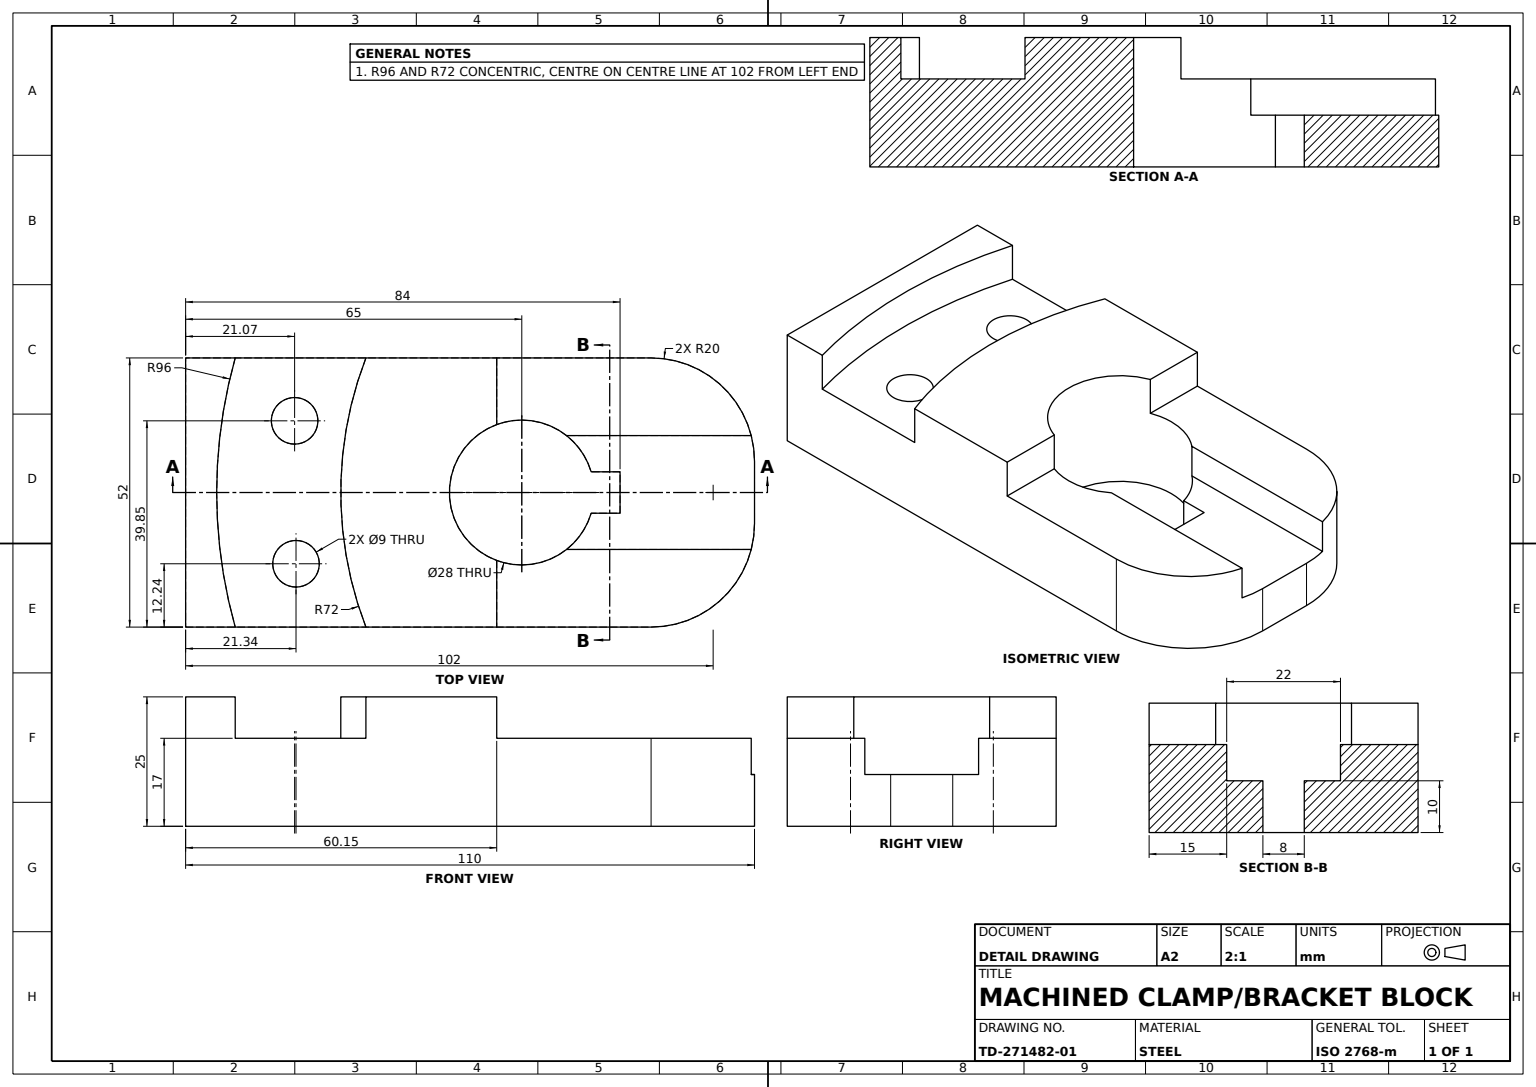
from build123d import *

# Parameters (mm, degrees)
BASE_OUTLINE_SKETCH_110X52_W      = 110
BASE_OUTLINE_SKETCH_110X52_H      = 52
BASE_BLOCK_25MM_DEPTH             = 12.5
SIDE_PROFILE_SKETCH_R             = 4.5
SIDE_PROFILE_CUT_THROUGH_75_DEPTH = 75
SIDE_PROFILE_CUT_8MM_DEPTH        = 8
SIDE_PROFILE_CUT_THROUGH_78_DEPTH = 78
SLOT_CUT_8MM_DEPTH                = 8
POCKET_CUT_15MM_DEPTH             = 15
END_FILLET_R20_R                  = 20


with BuildPart() as part:
    # Base Outline Sketch 110x52 → Base Block 25mm (new, symmetric)
    with BuildSketch(Plane(origin=(0, 0, 0), x_dir=(1, 0, 0), z_dir=(0, 1, 0))):
        with Locations((55, 0)):
            Rectangle(BASE_OUTLINE_SKETCH_110X52_W, BASE_OUTLINE_SKETCH_110X52_H)
    extrude(amount=BASE_BLOCK_25MM_DEPTH, both=True)

    # Side Profile Sketch → Side Profile Cut Through 75 (cut)
    with BuildSketch(Plane(origin=(0, 12.5, 0), x_dir=(1, 0, 0), z_dir=(0, 1, 0))):
        with Locations(Location((21.074107975, 13.849780556, 0), (0, 0, 270))):
            Circle(SIDE_PROFILE_SKETCH_R)
        with Locations(Location((21.343878228, -13.764722322, 0), (0, 0, 270))):
            Circle(SIDE_PROFILE_SKETCH_R)
    extrude(amount=-SIDE_PROFILE_CUT_THROUGH_75_DEPTH, mode=Mode.SUBTRACT)

    # Sketch2_6 → Side Profile Cut 8mm (cut)
    with BuildSketch(Plane(origin=(0, 12.5, 0), x_dir=(1, 0, 0), z_dir=(0, 1, 0))):
        with BuildLine():
            Line((9.587879583, 26), (34.858358674, 26))
            ThreePointArc((34.858358674, 26), (30, 0), (34.858358674, -26))
            Line((34.858358674, -26), (9.587879583, -26))
            ThreePointArc((9.587879583, -26), (6, 0), (9.587879583, 26))
        make_face()
    extrude(amount=-SIDE_PROFILE_CUT_8MM_DEPTH, mode=Mode.SUBTRACT)

    # Sketch2_9 → Side Profile Cut Through 78 (cut)
    with BuildSketch(Plane(origin=(0, 12.5, 0), x_dir=(1, 0, 0), z_dir=(0, 1, 0))):
        with BuildLine():
            Line((84, -4), (84, 4))
            Line((84, 4), (78.416407865, 4))
            ThreePointArc((78.416407865, 4), (51, 0), (78.416407865, -4))
            Line((78.416407865, -4), (84, -4))
        make_face()
    extrude(amount=-SIDE_PROFILE_CUT_THROUGH_78_DEPTH, mode=Mode.SUBTRACT)

    # Slot Sketch 22 → Slot Cut 8mm (cut)
    with BuildSketch(Plane(origin=(0, 12.5, 0), x_dir=(1, 0, 0), z_dir=(0, 1, 0))):
        with BuildLine():
            Line((60.152360051, 26), (60.152360051, 13.133940267))
            ThreePointArc((60.152360051, 13.133940267), (67.184589621, 13.828505638), (73.660254038, 11))
            Line((73.660254038, 11), (110, 11))
            Line((110, 11), (110, 26))
            Line((110, 26), (60.152360051, 26))
        make_face()
        with BuildLine():
            Line((73.660254038, -11), (110, -11))
            Line((110, -11), (110, -26))
            Line((110, -26), (60.152360051, -26))
            Line((60.152360051, -26), (60.152360051, -13.133940267))
            ThreePointArc((60.152360051, -13.133940267), (67.184589621, -13.828505638), (73.660254038, -11))
        make_face()
    extrude(amount=-SLOT_CUT_8MM_DEPTH, mode=Mode.SUBTRACT)

    # Pocket Sketch → Pocket Cut 15mm (cut)
    with BuildSketch(Plane(origin=(0, 12.5, 0), x_dir=(1, 0, 0), z_dir=(0, 1, 0))):
        with BuildLine():
            Line((110, 11), (73.660254038, 11))
            ThreePointArc((73.660254038, 11), (76.579928765, 7.86798893), (78.416407865, 4))
            Line((78.416407865, 4), (84, 4))
            Line((84, 4), (84, -4))
            Line((84, -4), (78.416407865, -4))
            ThreePointArc((78.416407865, -4), (76.579928765, -7.86798893), (73.660254038, -11))
            Line((73.660254038, -11), (110, -11))
            Line((110, -11), (110, 11))
        make_face()
    extrude(amount=-POCKET_CUT_15MM_DEPTH, mode=Mode.SUBTRACT)

    # End Fillet R20
    end_fillet_r20_edges = [part.edges().sort_by_distance(p)[0] for p in [
        (110, -4, -26),
        (110, -4, 26),
    ]]
    fillet(end_fillet_r20_edges, radius=END_FILLET_R20_R)


solid = part.part
